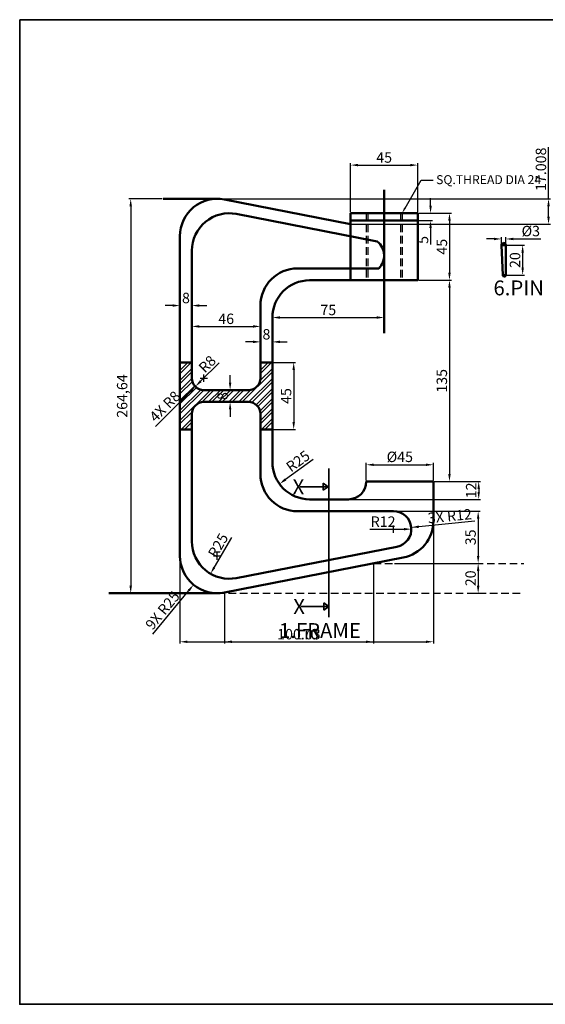
# Model space of a CAD drawing. Units: millimetres. Extents: x 210 to 1120, y -242 to 418.
# Tile 1 of 4: x 210 to 563, y -242 to 418. Entities that reach past the tile are written whole.
import ezdxf
from ezdxf import colors
from ezdxf.entities.mleader import LeaderData, LeaderLine
from ezdxf.math import Vec2, Vec3

# ---------------------------------------------------------------- set-up
doc = ezdxf.new("R2010")
doc.units = ezdxf.units.MM
doc.header["$LTSCALE"] = 0.4
doc.linetypes.add('DASHED', pattern=[19.05, 12.7, -6.35])
for name, color, linetype, lineweight in [('M-DIMS', 2, 'Continuous', 25), ('M-HATC', 8, 'Continuous', 18), ('M-HIDN', 4, 'DASHED', 25), ('M-OUTL', 7, 'Continuous', 50), ('M-SECT', 6, 'Continuous', 35), ('M-TEXT', 3, 'Continuous', 25), ('M-TTLB', 7, 'Continuous', 35)]:
    doc.layers.add(name, color=color, linetype=linetype, lineweight=lineweight)
doc.styles.get("Standard").update_dxf_attribs({"font": 'arial.ttf'})
doc.dimstyles.new('ISO-25', dxfattribs={"dimtxt": 7, "dimasz": 5, "dimexe": 1.25, "dimexo": 0.625, "dimtad": 1, "dimtxsty": 'Standard', "dimcen": 2.5, "dimadec": 0, "dimazin": 0, "dimtfac": 1, "dimtofl": 0, "dimtmove": 0, "dimatfit": 3, "dimfxl": 1, "dimarcsym": 0})

# ---------------------------------------------------------------- blocks, each defined once
blk = doc.blocks.new('*D1')
at = {"layer": 'Defpoints', "color": 0, "transparency": 16777216}
for p in [(350.72, 68.21), (338.22, 46.56)]:
    blk.add_point(p, dxfattribs=at)
at = {"layer": 'M-DIMS', "color": 0, "lineweight": -2, "transparency": 16777216}
blk.add_line((352.23, 70.83), (340.72, 50.89), dxfattribs=at)
at = {"layer": 'M-DIMS', "color": 0, "transparency": 16777216}
blk.add_solid([(340, 51.31), (341.44, 50.47), (338.22, 46.56)], dxfattribs=at)
at = {"layer": 'M-DIMS', "color": 0, "transparency": 16777216, "insert": (344.09, 65.13), "char_height": 7, "attachment_point": 5, "rotation": 60}
blk.add_mtext('R25', dxfattribs=at)
blk = doc.blocks.new('*D2')
at = {"layer": 'Defpoints', "color": 0, "transparency": 16777216}
for p in [(404.72, 121.5), (384.46, 106.85)]:
    blk.add_point(p, dxfattribs=at)
at = {"layer": 'M-DIMS', "color": 0, "lineweight": -2, "transparency": 16777216}
blk.add_line((407.17, 123.27), (388.51, 109.78), dxfattribs=at)
at = {"layer": 'M-DIMS', "color": 0, "transparency": 16777216}
blk.add_solid([(388.02, 110.45), (389, 109.1), (384.46, 106.85)], dxfattribs=at)
at = {"layer": 'M-DIMS', "color": 0, "transparency": 16777216, "insert": (397.41, 121.39), "char_height": 7, "attachment_point": 5, "rotation": 35.87577}
blk.add_mtext('R25', dxfattribs=at)
blk = doc.blocks.new('*D3')
at = {"layer": 'Defpoints', "color": 0, "transparency": 16777216}
for p in [(460.96, 76.5), (472.96, 76.5)]:
    blk.add_point(p, dxfattribs=at)
at = {"layer": 'M-DIMS', "color": 0, "lineweight": -2, "transparency": 16777216}
blk.add_line((445.06, 76.5), (467.96, 76.5), dxfattribs=at)
at = {"layer": 'M-DIMS', "color": 0, "transparency": 16777216}
blk.add_solid([(467.96, 77.33), (467.96, 75.66), (472.96, 76.5)], dxfattribs=at)
at = {"layer": 'M-DIMS', "color": 0, "transparency": 16777216, "insert": (454.01, 80.64), "char_height": 7, "attachment_point": 5}
blk.add_mtext('R12', dxfattribs=at)
blk = doc.blocks.new('*D4')
at = {"layer": 'Defpoints', "color": 0, "transparency": 16777216}
for p in [(328.02, 172.2), (333.72, 177.82)]:
    blk.add_point(p, dxfattribs=at)
at = {"layer": 'M-DIMS', "color": 0, "lineweight": -2, "transparency": 16777216}
blk.add_line((344.08, 188.04), (331.58, 175.71), dxfattribs=at)
at = {"layer": 'M-DIMS', "color": 0, "transparency": 16777216}
blk.add_solid([(331, 176.31), (332.17, 175.12), (328.02, 172.2)], dxfattribs=at)
at = {"layer": 'M-DIMS', "color": 0, "transparency": 16777216, "insert": (336.66, 186.62), "char_height": 7, "attachment_point": 5, "rotation": 44.59101}
blk.add_mtext('R8', dxfattribs=at)
blk = doc.blocks.new('*D5')
at = {"layer": 'Defpoints', "color": 0, "transparency": 16777216}
for p in [(306.33, 298.14), (284.66, 33.5), (306.33, 33.5)]:
    blk.add_point(p, dxfattribs=at)
at = {"layer": 'M-DIMS', "color": 0, "lineweight": -2, "transparency": 16777216}
for p, q in [((305.7, 298.14), (283.41, 298.14)), ((284.66, 293.14), (284.66, 38.5)), ((305.7, 33.5), (283.41, 33.5))]:
    blk.add_line(p, q, dxfattribs=at)
at = {"layer": 'M-DIMS', "color": 0, "transparency": 16777216}
for points in [[(283.82, 293.14), (285.49, 293.14), (284.66, 298.14)], [(283.82, 38.5), (285.49, 38.5), (284.66, 33.5)]]:
    blk.add_solid(points, dxfattribs=at)
at = {"layer": 'M-DIMS', "color": 0, "transparency": 16777216, "insert": (279.82, 165.82), "char_height": 7, "attachment_point": 5, "rotation": 90}
blk.add_mtext('264,64', dxfattribs=at)
blk = doc.blocks.new('*D6')
at = {"layer": 'Defpoints', "color": 0, "transparency": 16777216}
for p in [(317.72, 226.51), (325.72, 226.51), (325.72, 226.51)]:
    blk.add_point(p, dxfattribs=at)
at = {"layer": 'M-DIMS', "color": 0, "lineweight": -2, "transparency": 16777216}
for p, q in [((312.72, 226.51), (307.72, 226.51)), ((317.72, 227.14), (317.72, 227.76)), ((325.72, 227.14), (325.72, 227.76)), ((330.72, 226.51), (335.72, 226.51))]:
    blk.add_line(p, q, dxfattribs=at)
at = {"layer": 'M-DIMS', "color": 0, "transparency": 16777216}
for points in [[(312.72, 227.35), (312.72, 225.68), (317.72, 226.51)], [(330.72, 227.35), (330.72, 225.68), (325.72, 226.51)]]:
    blk.add_solid(points, dxfattribs=at)
at = {"layer": 'M-DIMS', "color": 0, "transparency": 16777216, "insert": (321.72, 230.71), "char_height": 7, "attachment_point": 5}
blk.add_mtext('8', dxfattribs=at)
blk = doc.blocks.new('*D7')
at = {"layer": 'Defpoints', "color": 0, "transparency": 16777216}
for p in [(371.72, 212.54), (325.72, 209.96), (371.72, 209.96)]:
    blk.add_point(p, dxfattribs=at)
at = {"layer": 'M-DIMS', "color": 0, "lineweight": -2, "transparency": 16777216}
for p, q in [((325.72, 210.58), (325.72, 213.79)), ((330.72, 212.54), (366.72, 212.54)), ((371.72, 210.58), (371.72, 213.79))]:
    blk.add_line(p, q, dxfattribs=at)
at = {"layer": 'M-DIMS', "color": 0, "transparency": 16777216}
for points in [[(330.72, 213.37), (330.72, 211.7), (325.72, 212.54)], [(366.72, 213.37), (366.72, 211.7), (371.72, 212.54)]]:
    blk.add_solid(points, dxfattribs=at)
at = {"layer": 'M-DIMS', "color": 0, "transparency": 16777216, "insert": (348.72, 216.74), "char_height": 7, "attachment_point": 5}
blk.add_mtext('46', dxfattribs=at)
blk = doc.blocks.new('*D8')
at = {"layer": 'Defpoints', "color": 0, "transparency": 16777216}
for p in [(371.72, 202.16), (379.72, 202.16), (379.72, 202.16)]:
    blk.add_point(p, dxfattribs=at)
at = {"layer": 'M-DIMS', "color": 0, "lineweight": -2, "transparency": 16777216}
for p, q in [((366.72, 202.16), (361.72, 202.16)), ((371.72, 202.78), (371.72, 203.41)), ((379.72, 202.78), (379.72, 203.41)), ((384.72, 202.16), (389.72, 202.16))]:
    blk.add_line(p, q, dxfattribs=at)
at = {"layer": 'M-DIMS', "color": 0, "transparency": 16777216}
for points in [[(366.72, 202.99), (366.72, 201.33), (371.72, 202.16)], [(384.72, 202.99), (384.72, 201.33), (379.72, 202.16)]]:
    blk.add_solid(points, dxfattribs=at)
at = {"layer": 'M-DIMS', "color": 0, "transparency": 16777216, "insert": (375.72, 206.36), "char_height": 7, "attachment_point": 5}
blk.add_mtext('8', dxfattribs=at)
blk = doc.blocks.new('*D9')
at = {"layer": 'Defpoints', "color": 0, "transparency": 16777216}
for p in [(379.72, 188.32), (379.72, 143.32), (394.01, 143.32)]:
    blk.add_point(p, dxfattribs=at)
at = {"layer": 'M-DIMS', "color": 0, "lineweight": -2, "transparency": 16777216}
for p, q in [((380.34, 188.32), (395.26, 188.32)), ((394.01, 183.32), (394.01, 148.32)), ((380.34, 143.32), (395.26, 143.32))]:
    blk.add_line(p, q, dxfattribs=at)
at = {"layer": 'M-DIMS', "color": 0, "transparency": 16777216}
for points in [[(393.18, 183.32), (394.85, 183.32), (394.01, 188.32)], [(393.18, 148.32), (394.85, 148.32), (394.01, 143.32)]]:
    blk.add_solid(points, dxfattribs=at)
at = {"layer": 'M-DIMS', "color": 0, "transparency": 16777216, "insert": (389.83, 165.82), "char_height": 7, "attachment_point": 5, "rotation": 90}
blk.add_mtext('45', dxfattribs=at)
blk = doc.blocks.new('*D10')
at = {"layer": 'Defpoints', "color": 0, "transparency": 16777216}
for p in [(348.72, 169.82), (348.72, 161.82), (351.36, 161.82)]:
    blk.add_point(p, dxfattribs=at)
at = {"layer": 'M-DIMS', "color": 0, "lineweight": -2, "transparency": 16777216}
for p, q in [((351.36, 174.82), (351.36, 179.82)), ((349.34, 169.82), (352.61, 169.82)), ((349.34, 161.82), (352.61, 161.82)), ((351.36, 156.82), (351.36, 151.82))]:
    blk.add_line(p, q, dxfattribs=at)
at = {"layer": 'M-DIMS', "color": 0, "transparency": 16777216}
for points in [[(350.52, 174.82), (352.19, 174.82), (351.36, 169.82)], [(350.52, 156.82), (352.19, 156.82), (351.36, 161.82)]]:
    blk.add_solid(points, dxfattribs=at)
at = {"layer": 'M-DIMS', "color": 0, "transparency": 16777216, "insert": (347.16, 165.82), "char_height": 7, "attachment_point": 5, "rotation": 90}
blk.add_mtext('8', dxfattribs=at)
blk = doc.blocks.new('*D11')
at = {"layer": 'Defpoints', "color": 0, "transparency": 16777216}
for p in [(379.72, 218.5), (454.72, 218.5), (454.72, 218.5)]:
    blk.add_point(p, dxfattribs=at)
at = {"layer": 'M-DIMS', "color": 0, "lineweight": -2, "transparency": 16777216}
for p, q in [((379.72, 219.12), (379.72, 219.75)), ((384.72, 218.5), (449.72, 218.5)), ((454.72, 219.12), (454.72, 219.75))]:
    blk.add_line(p, q, dxfattribs=at)
at = {"layer": 'M-DIMS', "color": 0, "transparency": 16777216}
for points in [[(384.72, 219.33), (384.72, 217.66), (379.72, 218.5)], [(449.72, 219.33), (449.72, 217.66), (454.72, 218.5)]]:
    blk.add_solid(points, dxfattribs=at)
at = {"layer": 'M-DIMS', "color": 0, "transparency": 16777216, "insert": (417.22, 222.68), "char_height": 7, "attachment_point": 5}
blk.add_mtext('75', dxfattribs=at)
blk = doc.blocks.new('*D12')
at = {"layer": 'Defpoints', "color": 0, "transparency": 16777216}
for p in [(477.22, 288.5), (477.22, 243.5), (498.54, 243.5)]:
    blk.add_point(p, dxfattribs=at)
at = {"layer": 'M-DIMS', "color": 0, "lineweight": -2, "transparency": 16777216}
for p, q in [((477.84, 288.5), (499.79, 288.5)), ((498.54, 283.5), (498.54, 248.5)), ((477.84, 243.5), (499.79, 243.5))]:
    blk.add_line(p, q, dxfattribs=at)
at = {"layer": 'M-DIMS', "color": 0, "transparency": 16777216}
for points in [[(497.7, 283.5), (499.37, 283.5), (498.54, 288.5)], [(497.7, 248.5), (499.37, 248.5), (498.54, 243.5)]]:
    blk.add_solid(points, dxfattribs=at)
at = {"layer": 'M-DIMS', "color": 0, "transparency": 16777216, "insert": (494.35, 266), "char_height": 7, "attachment_point": 5, "rotation": 90}
blk.add_mtext('45', dxfattribs=at)
blk = doc.blocks.new('*D13')
at = {"layer": 'Defpoints', "color": 0, "transparency": 16777216}
for p in [(487.72, 119.69), (442.72, 108.5), (487.72, 108.5)]:
    blk.add_point(p, dxfattribs=at)
at = {"layer": 'M-DIMS', "color": 0, "lineweight": -2, "transparency": 16777216}
for p, q in [((442.72, 109.12), (442.72, 120.94)), ((447.72, 119.69), (482.72, 119.69)), ((487.72, 109.12), (487.72, 120.94))]:
    blk.add_line(p, q, dxfattribs=at)
at = {"layer": 'M-DIMS', "color": 0, "transparency": 16777216}
for points in [[(447.72, 120.52), (447.72, 118.86), (442.72, 119.69)], [(482.72, 120.52), (482.72, 118.86), (487.72, 119.69)]]:
    blk.add_solid(points, dxfattribs=at)
at = {"layer": 'M-DIMS', "color": 0, "transparency": 16777216, "insert": (465.22, 124.09), "char_height": 7, "attachment_point": 5}
blk.add_mtext('%%C45', dxfattribs=at)
blk = doc.blocks.new('*D14')
at = {"layer": 'Defpoints', "color": 0, "transparency": 16777216}
for p in [(487.72, 108.5), (417.72, 96.5), (518.15, 96.5)]:
    blk.add_point(p, dxfattribs=at)
at = {"layer": 'M-DIMS', "color": 0, "lineweight": -2, "transparency": 16777216}
for p, q in [((488.34, 108.5), (519.4, 108.5)), ((518.15, 103.5), (518.15, 101.5)), ((418.34, 96.5), (519.4, 96.5))]:
    blk.add_line(p, q, dxfattribs=at)
at = {"layer": 'M-DIMS', "color": 0, "transparency": 16777216}
for points in [[(517.32, 103.5), (518.98, 103.5), (518.15, 108.5)], [(517.32, 101.5), (518.98, 101.5), (518.15, 96.5)]]:
    blk.add_solid(points, dxfattribs=at)
at = {"layer": 'M-DIMS', "color": 0, "transparency": 16777216, "insert": (514.01, 102.5), "char_height": 7, "attachment_point": 5, "rotation": 90}
blk.add_mtext('12', dxfattribs=at)
blk = doc.blocks.new('*D15')
at = {"layer": 'Defpoints', "color": 0, "transparency": 16777216}
for p in [(511.06, 53.5), (511.06, 33.5), (517.8, 33.5)]:
    blk.add_point(p, dxfattribs=at)
at = {"layer": 'M-DIMS', "color": 0, "lineweight": -2, "transparency": 16777216}
for p, q in [((511.68, 53.5), (519.05, 53.5)), ((517.8, 48.5), (517.8, 38.5)), ((511.68, 33.5), (519.05, 33.5))]:
    blk.add_line(p, q, dxfattribs=at)
at = {"layer": 'M-DIMS', "color": 0, "transparency": 16777216}
for points in [[(516.96, 48.5), (518.63, 48.5), (517.8, 53.5)], [(516.96, 38.5), (518.63, 38.5), (517.8, 33.5)]]:
    blk.add_solid(points, dxfattribs=at)
at = {"layer": 'M-DIMS', "color": 0, "transparency": 16777216, "insert": (513.6, 43.5), "char_height": 7, "attachment_point": 5, "rotation": 90}
blk.add_mtext('20', dxfattribs=at)
blk = doc.blocks.new('*D16')
at = {"layer": 'Defpoints', "color": 0, "transparency": 16777216}
for p in [(460.96, 88.5), (460.96, 53.5), (517.8, 53.5)]:
    blk.add_point(p, dxfattribs=at)
at = {"layer": 'M-DIMS', "color": 0, "lineweight": -2, "transparency": 16777216}
for p, q in [((461.59, 88.5), (519.05, 88.5)), ((517.8, 83.5), (517.8, 58.5)), ((461.59, 53.5), (519.05, 53.5))]:
    blk.add_line(p, q, dxfattribs=at)
at = {"layer": 'M-DIMS', "color": 0, "transparency": 16777216}
for points in [[(516.96, 83.5), (518.63, 83.5), (517.8, 88.5)], [(516.96, 58.5), (518.63, 58.5), (517.8, 53.5)]]:
    blk.add_solid(points, dxfattribs=at)
at = {"layer": 'M-DIMS', "color": 0, "transparency": 16777216, "insert": (513.6, 71), "char_height": 7, "attachment_point": 5, "rotation": 90}
blk.add_mtext('35', dxfattribs=at)
blk = doc.blocks.new('*D17')
at = {"layer": 'Defpoints', "color": 0, "transparency": 16777216}
for p in [(488.81, 243.5), (488.81, 108.5), (498.54, 108.5)]:
    blk.add_point(p, dxfattribs=at)
at = {"layer": 'M-DIMS', "color": 0, "lineweight": -2, "transparency": 16777216}
for p, q in [((489.44, 243.5), (499.79, 243.5)), ((498.54, 238.5), (498.54, 113.5)), ((489.44, 108.5), (499.79, 108.5))]:
    blk.add_line(p, q, dxfattribs=at)
at = {"layer": 'M-DIMS', "color": 0, "transparency": 16777216}
for points in [[(497.7, 238.5), (499.37, 238.5), (498.54, 243.5)], [(497.7, 113.5), (499.37, 113.5), (498.54, 108.5)]]:
    blk.add_solid(points, dxfattribs=at)
at = {"layer": 'M-DIMS', "color": 0, "transparency": 16777216, "insert": (494.33, 176), "char_height": 7, "attachment_point": 5, "rotation": 90}
blk.add_mtext('135', dxfattribs=at)
blk = doc.blocks.new('*D20')
at = {"layer": 'Defpoints', "color": 0, "transparency": 16777216}
for p in [(477.22, 288.5), (477.22, 283.5), (485.85, 283.5)]:
    blk.add_point(p, dxfattribs=at)
at = {"layer": 'M-DIMS', "color": 0, "lineweight": -2, "transparency": 16777216}
for p, q in [((485.85, 293.5), (485.85, 298.5)), ((477.84, 288.5), (487.1, 288.5)), ((477.84, 283.5), (487.1, 283.5)), ((485.85, 278.5), (485.85, 267.61))]:
    blk.add_line(p, q, dxfattribs=at)
at = {"layer": 'M-DIMS', "color": 0, "transparency": 16777216}
for points in [[(485.02, 293.5), (486.68, 293.5), (485.85, 288.5)], [(485.02, 278.5), (486.68, 278.5), (485.85, 283.5)]]:
    blk.add_solid(points, dxfattribs=at)
at = {"layer": 'M-DIMS', "color": 0, "transparency": 16777216, "insert": (481.67, 270.55), "char_height": 7, "attachment_point": 5, "rotation": 90}
blk.add_mtext('5', dxfattribs=at)
blk = doc.blocks.new('*D43')
at = {"layer": 'Defpoints', "color": 0, "ltscale": 0.4, "transparency": 16777216}
for p in [(534.88, 267.02), (535.38, 247.02), (547.64, 247.02)]:
    blk.add_point(p, dxfattribs=at)
at = {"layer": 'M-DIMS', "color": 0, "lineweight": -2, "ltscale": 0.4, "transparency": 16777216}
for p, q in [((535.51, 267.02), (548.89, 267.02)), ((547.64, 262.02), (547.64, 252.02)), ((536.01, 247.02), (548.89, 247.02))]:
    blk.add_line(p, q, dxfattribs=at)
at = {"layer": 'M-DIMS', "color": 0, "ltscale": 0.4, "transparency": 16777216}
for points in [[(546.81, 262.02), (548.48, 262.02), (547.64, 267.02)], [(546.81, 252.02), (548.48, 252.02), (547.64, 247.02)]]:
    blk.add_solid(points, dxfattribs=at)
at = {"layer": 'M-DIMS', "color": 0, "ltscale": 0.4, "transparency": 16777216, "insert": (543.44, 257.02), "char_height": 7, "attachment_point": 5, "rotation": 90}
blk.add_mtext('20', dxfattribs=at)
blk = doc.blocks.new('*D44')
at = {"layer": 'Defpoints', "color": 0, "ltscale": 0.4, "transparency": 16777216}
for p in [(536.38, 271.22), (533.38, 267.02), (536.38, 267.02)]:
    blk.add_point(p, dxfattribs=at)
at = {"layer": 'M-DIMS', "color": 0, "lineweight": -2, "ltscale": 0.4, "transparency": 16777216}
for p, q in [((528.38, 271.22), (523.38, 271.22)), ((533.38, 267.65), (533.38, 272.47)), ((536.38, 267.65), (536.38, 272.47)), ((541.38, 271.22), (559.84, 271.22))]:
    blk.add_line(p, q, dxfattribs=at)
at = {"layer": 'M-DIMS', "color": 0, "ltscale": 0.4, "transparency": 16777216}
for points in [[(528.38, 272.05), (528.38, 270.38), (533.38, 271.22)], [(541.38, 272.05), (541.38, 270.38), (536.38, 271.22)]]:
    blk.add_solid(points, dxfattribs=at)
at = {"layer": 'M-DIMS', "color": 0, "ltscale": 0.4, "transparency": 16777216, "insert": (553.11, 275.61), "char_height": 7, "attachment_point": 5}
blk.add_mtext('%%C3', dxfattribs=at)
blk = doc.blocks.new('SECTION-ARROW')
for p, q in [((0, 2.43), (18.69, 2.43)), ((15.48, 2.43), (15.48, 4.85)), ((15.48, 4.85), (18.69, 2.43)), ((15.48, 2.43), (15.48, 0)), ((15.48, 0), (18.69, 2.43))]:
    blk.add_line(p, q)
blk = doc.blocks.new('*D46')
at = {"layer": 'Defpoints', "color": 0, "ltscale": 0.4, "transparency": 16777216}
for p in [(487.72, 108.5), (317.72, 58.5), (487.72, 0.92)]:
    blk.add_point(p, dxfattribs=at)
at = {"layer": 'M-DIMS', "color": 0, "lineweight": -2, "ltscale": 0.4, "transparency": 16777216}
for p, q in [((487.72, 107.87), (487.72, -0.33)), ((317.72, 57.87), (317.72, -0.33)), ((322.72, 0.92), (482.72, 0.92))]:
    blk.add_line(p, q, dxfattribs=at)
at = {"layer": 'M-DIMS', "color": 0, "ltscale": 0.4, "transparency": 16777216}
for points in [[(322.72, 1.75), (322.72, 0.08), (317.72, 0.92)], [(482.72, 1.75), (482.72, 0.08), (487.72, 0.92)]]:
    blk.add_solid(points, dxfattribs=at)
at = {"layer": 'M-DIMS', "color": 0, "ltscale": 0.4, "transparency": 16777216, "insert": (402.72, 5.12), "char_height": 7, "attachment_point": 5}
blk.add_mtext('170', dxfattribs=at)
blk = doc.blocks.new('*D47')
at = {"layer": 'Defpoints', "color": 0, "ltscale": 0.4, "transparency": 16777216}
for p in [(477.22, 320.78), (432.22, 288.5), (477.22, 288.5)]:
    blk.add_point(p, dxfattribs=at)
at = {"layer": 'M-DIMS', "color": 0, "lineweight": -2, "ltscale": 0.4, "transparency": 16777216}
for p, q in [((432.22, 289.12), (432.22, 322.03)), ((437.22, 320.78), (472.22, 320.78)), ((477.22, 289.12), (477.22, 322.03))]:
    blk.add_line(p, q, dxfattribs=at)
at = {"layer": 'M-DIMS', "color": 0, "ltscale": 0.4, "transparency": 16777216}
for points in [[(437.22, 321.62), (437.22, 319.95), (432.22, 320.78)], [(472.22, 321.62), (472.22, 319.95), (477.22, 320.78)]]:
    blk.add_solid(points, dxfattribs=at)
at = {"layer": 'M-DIMS', "color": 0, "ltscale": 0.4, "transparency": 16777216, "insert": (454.72, 324.97), "char_height": 7, "attachment_point": 5}
blk.add_mtext('45', dxfattribs=at)
blk = doc.blocks.new('*D48')
at = {"layer": 'Defpoints', "color": 0, "ltscale": 0.4, "transparency": 16777216}
for p in [(342.72, 298.14), (565, 298.14), (432.22, 281.13)]:
    blk.add_point(p, dxfattribs=at)
at = {"layer": 'M-DIMS', "color": 0, "lineweight": -2, "ltscale": 0.4, "transparency": 16777216}
for p, q in [((565, 298.14), (565, 332.81)), ((343.34, 298.14), (566.25, 298.14)), ((565, 286.13), (565, 293.14)), ((432.84, 281.13), (566.25, 281.13))]:
    blk.add_line(p, q, dxfattribs=at)
at = {"layer": 'M-DIMS', "color": 0, "ltscale": 0.4, "transparency": 16777216}
for points in [[(564.16, 293.14), (565.83, 293.14), (565, 298.14)], [(564.16, 286.13), (565.83, 286.13), (565, 281.13)]]:
    blk.add_solid(points, dxfattribs=at)
at = {"layer": 'M-DIMS', "color": 0, "ltscale": 0.4, "transparency": 16777216, "insert": (560.8, 317.98), "char_height": 7, "attachment_point": 5, "rotation": 90}
blk.add_mtext('17.008', dxfattribs=at)
blk = doc.blocks.new('*D49')
at = {"layer": 'Defpoints', "color": 0, "ltscale": 0.4, "transparency": 16777216}
for p in [(447.54, 53.5), (347.51, 33.96), (447.54, 0.92)]:
    blk.add_point(p, dxfattribs=at)
at = {"layer": 'M-DIMS', "color": 0, "lineweight": -2, "ltscale": 0.4, "transparency": 16777216}
for p, q in [((447.54, 52.87), (447.54, -0.33)), ((347.51, 33.34), (347.51, -0.33)), ((352.51, 0.92), (442.54, 0.92))]:
    blk.add_line(p, q, dxfattribs=at)
at = {"layer": 'M-DIMS', "color": 0, "ltscale": 0.4, "transparency": 16777216}
for points in [[(352.51, 1.75), (352.51, 0.08), (347.51, 0.92)], [(442.54, 1.75), (442.54, 0.08), (447.54, 0.92)]]:
    blk.add_solid(points, dxfattribs=at)
at = {"layer": 'M-DIMS', "color": 0, "ltscale": 0.4, "transparency": 16777216, "insert": (397.52, 5.12), "char_height": 7, "attachment_point": 5}
blk.add_mtext('100.03', dxfattribs=at)
blk = doc.blocks.new('*D54')
at = {"layer": 'Defpoints', "color": 0, "ltscale": 0.4, "transparency": 16777216}
for p in [(342.72, 58.5), (326.83, 39.2)]:
    blk.add_point(p, dxfattribs=at)
at = {"layer": 'M-DIMS', "color": 0, "lineweight": -2, "ltscale": 0.4, "transparency": 16777216}
for p, q in [((342.72, 56), (342.72, 61)), ((340.22, 58.5), (345.22, 58.5)), ((299.45, 5.95), (323.65, 35.34))]:
    blk.add_line(p, q, dxfattribs=at)
at = {"layer": 'M-DIMS', "color": 0, "ltscale": 0.4, "transparency": 16777216}
blk.add_solid([(323, 35.87), (324.29, 34.81), (326.83, 39.2)], dxfattribs=at)
at = {"layer": 'M-DIMS', "color": 0, "ltscale": 0.4, "transparency": 16777216, "insert": (306.72, 21.39), "char_height": 7, "attachment_point": 5, "rotation": 50.52629}
blk.add_mtext('9X R25', dxfattribs=at)
blk = doc.blocks.new('*D55')
at = {"layer": 'Defpoints', "color": 0, "ltscale": 0.4, "transparency": 16777216}
for p in [(460.96, 76.5), (472.91, 77.65)]:
    blk.add_point(p, dxfattribs=at)
at = {"layer": 'M-DIMS', "color": 0, "lineweight": -2, "ltscale": 0.4, "transparency": 16777216}
for p, q in [((515.65, 81.79), (477.88, 78.13)), ((458.46, 76.5), (463.46, 76.5)), ((460.96, 74), (460.96, 79))]:
    blk.add_line(p, q, dxfattribs=at)
at = {"layer": 'M-DIMS', "color": 0, "ltscale": 0.4, "transparency": 16777216}
blk.add_solid([(477.8, 78.96), (477.96, 77.3), (472.91, 77.65)], dxfattribs=at)
at = {"layer": 'M-DIMS', "color": 0, "ltscale": 0.4, "transparency": 16777216, "insert": (498.85, 84.38), "char_height": 7, "attachment_point": 5, "rotation": 5.52485}
blk.add_mtext('3X R12', dxfattribs=at)
blk = doc.blocks.new('*D56')
at = {"layer": 'Defpoints', "color": 0, "ltscale": 0.4, "transparency": 16777216}
for p in [(328.06, 172.16), (333.72, 177.82)]:
    blk.add_point(p, dxfattribs=at)
at = {"layer": 'M-DIMS', "color": 0, "lineweight": -2, "ltscale": 0.4, "transparency": 16777216}
for p, q in [((333.72, 175.32), (333.72, 180.32)), ((331.22, 177.82), (336.22, 177.82)), ((301.28, 145.38), (324.53, 168.63))]:
    blk.add_line(p, q, dxfattribs=at)
at = {"layer": 'M-DIMS', "color": 0, "ltscale": 0.4, "transparency": 16777216}
blk.add_solid([(323.94, 169.22), (325.12, 168.04), (328.06, 172.16)], dxfattribs=at)
at = {"layer": 'M-DIMS', "color": 0, "ltscale": 0.4, "transparency": 16777216, "insert": (308.17, 158.21), "char_height": 7, "attachment_point": 5, "rotation": 45.00087}
blk.add_mtext('4X R8', dxfattribs=at)

msp = doc.modelspace()

# ---------------------------------------------------------------- hatches: boundary and pattern name
at = {"layer": 'M-HATC'}
h = msp.add_hatch(dxfattribs=at)
h.set_pattern_fill('ANSI32', color=256, scale=0.5)
h.paths.add_polyline_path([(379.7189, 188.3201), (371.7189, 188.3201), (371.7189, 177.8201, -0.41421356), (363.7189, 169.8201), (333.7189, 169.8201, -0.41421356), (325.7189, 177.8201), (325.7189, 188.3201), (317.7189, 188.3201), (317.7189, 165.8201), (317.7189, 143.3201), (325.7189, 143.3201), (325.7189, 153.8201, -0.41421356), (333.7189, 161.8201), (363.7189, 161.8201, -0.41421356), (371.7189, 153.8201), (371.7189, 143.3201), (379.7189, 143.3201), (379.7189, 165.8201)])

# ---------------------------------------------------------------- linework, layer by layer
at = {"layer": 'M-HIDN'}
for p, q in [((442.7189, 288.4977), (442.7189, 243.4977)), ((443.7189, 288.4977), (443.7189, 243.4977)), ((465.7189, 288.4977), (465.7189, 243.4977)), ((466.7189, 288.4977), (466.7189, 243.4977)), ((447.5374, 53.4977), (548.4982, 53.4977)), ((342.7189, 33.4977), (548.3926, 33.4977))]:
    msp.add_line(p, q, dxfattribs=at)
at = {"layer": 'M-OUTL'}
for p, q in [((454.7189, 208.0107), (454.7189, 304.2823)), ((342.7189, 298.1425), (306.3276, 298.1425)), ((432.2189, 281.1344), (347.5112, 297.6789)), ((450.1236, 269.4862), (355.5112, 287.9652)), ((477.2189, 288.4977), (432.2189, 288.4977)), ((432.2189, 288.4977), (432.2189, 243.4977)), ((454.7189, 288.4977), (454.7189, 243.4977)), ((477.2189, 243.4977), (477.2189, 288.4977)), ((477.2189, 283.4977), (432.2189, 283.4977)), ((454.7189, 278.4977), (454.7189, 283.4977)), ((317.7189, 165.8201), (317.7189, 273.1425)), ((325.7189, 177.8201), (325.7189, 263.4288)), ((396.7189, 251.4977), (451.1435, 251.4977)), ((404.7189, 243.4977), (477.2189, 243.4977)), ((432.2189, 243.4977), (477.2189, 243.4977)), ((371.7189, 177.8201), (371.7189, 226.4977)), ((379.7189, 165.8201), (379.7189, 218.4977)), ((317.7189, 188.3201), (325.7189, 188.3201)), ((371.7189, 188.3201), (379.7189, 188.3201)), ((317.7189, 165.8201), (317.7189, 58.4977)), ((333.7189, 169.8201), (363.7189, 169.8201)), ((379.7189, 165.8201), (379.7189, 121.4977)), ((333.7189, 161.8201), (363.7189, 161.8201)), ((325.7189, 153.8201), (325.7189, 68.2113)), ((371.7189, 153.8201), (371.7189, 113.4977)), ((317.7189, 143.3201), (325.7189, 143.3201)), ((371.7189, 143.3201), (379.7189, 143.3201)), ((442.7189, 108.4977), (487.7189, 108.4977)), ((487.7189, 81.9352), (487.7189, 108.4977)), ((404.7189, 96.4977), (430.7189, 96.4977)), ((396.7189, 88.4977), (460.9626, 88.4977)), ((463.2629, 64.7202), (355.5112, 43.6749)), ((467.5112, 57.3988), (347.5112, 33.9613)), ((342.7189, 33.4977), (270.0229, 33.4977))]:
    msp.add_line(p, q, dxfattribs=at)
at = {"layer": 'M-OUTL', "ltscale": 0.4}
for p, q in [((536.3815, 267.0225), (533.3815, 267.0225)), ((534.3815, 247.0225), (533.3815, 267.0225)), ((536.3815, 267.0225), (536.3815, 247.0225)), ((536.3815, 247.0225), (534.3815, 247.0225))]:
    msp.add_line(p, q, dxfattribs=at)
at = {"layer": 'M-OUTL'}
for centre, radius, start, end in [((342.7189, 273.1425), 25, 78.948543, 180), ((350.7189, 263.4288), 25, 78.948543, 180), ((442.7189, 260.0432), 12, 314.5918306, 51.8986166), ((396.7189, 226.4977), 25, 90, 180), ((404.7189, 218.4977), 25, 90, 180), ((333.7189, 177.8201), 8, 180, 270), ((363.7189, 177.8201), 8, 270, 0), ((333.7189, 153.8201), 8, 90, 180), ((363.7189, 153.8201), 8, 0, 90), ((404.7189, 121.4977), 25, 180, 270), ((396.7189, 113.4977), 25, 180, 270), ((430.7189, 108.4977), 12, 270, 360), ((460.9626, 76.4977), 12, 281.051457, 90), ((462.7189, 81.9352), 25, 281.051457, 0), ((350.7189, 68.2113), 25, 180, 281.051457), ((342.7189, 58.4977), 25, 180, 281.051457)]:
    msp.add_arc(centre, radius, start, end, dxfattribs=at)
at = {"layer": 'M-OUTL', "ltscale": 0.4}
for centre, radius, start, end in [((534.8815, 267.0225), 1.5, 0, 185.7248105), ((535.3815, 247.0225), 1, 180, 0)]:
    msp.add_arc(centre, radius, start, end, dxfattribs=at)
at = {"layer": 'M-SECT'}
msp.add_line((417.5578, 117.2772), (417.5578, 17.4177), dxfattribs=at)
at = {"layer": 'M-TTLB', "ltscale": 0.4}
msp.add_lwpolyline([(210.1659, 418.3486), (1119.5264, 418.3486), (1119.5264, -242.3444), (210.1659, -242.3444)], close=True, dxfattribs=at)

# ---------------------------------------------------------------- block references
at = {"layer": 'M-SECT'}
for p in [(398.3688, 102.5602), (398.863, 22.225)]:
    msp.add_blockref('SECTION-ARROW', p, dxfattribs=at)

# ---------------------------------------------------------------- texts
at = {"layer": 'M-TEXT', "attachment_point": 1}
for s, width, insert, char_height in [('\\pxqc;{\\H0.66667x;6.PIN} ', 102.502816, (493.7359, 243.3752), 15), ('X', 4.451993, (393.2632, 109.8473), 10), ('X', 4.451993, (393.7574, 29.5121), 10), ('\\pxqc;{\\H0.66667x;1.FRAME} ', 159.738723, (331.7515, 13.4299), 15)]:
    msp.add_mtext_dynamic_manual_height_columns(s, width=width, gutter_width=12.5, heights=[0], dxfattribs=dict(at, insert=insert, char_height=char_height))

# ---------------------------------------------------------------- dimensions: what is measured, and where the dimension line sits
at = {"layer": 'M-DIMS', "ltscale": 0.4}
for base, p1, p2, override, picture, middle in [((564.9982, 298.1425), (432.2189, 281.1344), (342.7189, 298.1425), {"dimdec": 3, "dimlfac": 1, "dimrnd": 0, "dimzin": 0, "dimdsep": 46, "dimlunit": 2}, '*D48', (560.7991, 317.9752)), ((547.642, 247.0225), (534.8815, 267.0225), (535.3815, 247.0225), {"dimclrd": 0, "dimclre": 0, "dimclrt": 0}, '*D43', (543.443, 257.0225))]:
    dim = msp.add_linear_dim(base=base, p1=p1, p2=p2, angle=90, dimstyle='ISO-25', override=override, dxfattribs=at)
    dim.commit()
    dim.dimension.update_dxf_attribs({"geometry": picture, "text_midpoint": middle})
for base, p1, p2, override, picture, middle in [((477.2189, 320.7823), (432.2189, 288.4977), (477.2189, 288.4977), {"dimdec": 0, "dimlfac": 1, "dimrnd": 0, "dimzin": 0, "dimdsep": 46, "dimlunit": 2}, '*D47', (454.7189, 324.967)), ((487.7189, 0.9177), (317.7189, 58.4977), (487.7189, 108.4977), {"dimdec": 0, "dimlfac": 1, "dimrnd": 0, "dimzin": 0, "dimdsep": 46, "dimlunit": 2}, '*D46', (402.7189, 5.1167)), ((447.5374, 0.9177), (347.5112, 33.9613), (447.5374, 53.4977), {"dimdec": 2, "dimlfac": 1, "dimrnd": 0, "dimzin": 0, "dimdsep": 46, "dimlunit": 2}, '*D49', (397.5243, 5.1191))]:
    dim = msp.add_linear_dim(base=base, p1=p1, p2=p2, dimstyle='ISO-25', override=override, dxfattribs=at)
    dim.commit()
    dim.dimension.update_dxf_attribs({"geometry": picture, "text_midpoint": middle})
at = {"layer": 'M-DIMS'}
for base, p1, p2, picture, middle in [((284.6552, 33.4977), (306.3276, 298.1425), (306.3276, 33.4977), '*D5', (279.8236, 165.8201)), ((485.8513, 283.4977), (477.2189, 288.4977), (477.2189, 283.4977), '*D20', (481.6666, 270.5521)), ((498.5354, 243.4977), (477.2189, 288.4977), (477.2189, 243.4977), '*D12', (494.3507, 265.9977)), ((498.5354, 108.4977), (488.8146, 243.4977), (488.8146, 108.4977), '*D17', (494.334, 175.9977)), ((394.0146, 143.3201), (379.7189, 188.3201), (379.7189, 143.3201), '*D9', (389.8299, 165.8201)), ((351.3552, 161.8201), (348.7189, 169.8201), (348.7189, 161.8201), '*D10', (347.1562, 165.8201)), ((518.1515, 96.4977), (487.7189, 108.4977), (417.7189, 96.4977), '*D14', (514.0122, 102.4977)), ((517.7965, 53.4977), (460.9626, 88.4977), (460.9626, 53.4977), '*D16', (513.5951, 70.9977)), ((517.7965, 33.4977), (511.0593, 53.4977), (511.0593, 33.4977), '*D15', (513.5975, 43.4977))]:
    dim = msp.add_linear_dim(base=base, p1=p1, p2=p2, angle=90, dimstyle='ISO-25', override={"dimclrd": 0, "dimclre": 0, "dimclrt": 0}, dxfattribs=at)
    dim.commit()
    dim.dimension.update_dxf_attribs({"geometry": picture, "text_midpoint": middle})
at = {"layer": 'M-DIMS', "ltscale": 0.4}
dim = msp.add_linear_dim(base=(536.3815, 271.2179), p1=(533.3815, 267.0225), p2=(536.3815, 267.0225), text='%%C<>', dimstyle='ISO-25', override={"dimclrd": 0, "dimclre": 0, "dimclrt": 0}, dxfattribs=at)
dim.commit()
dim.dimension.update_dxf_attribs({"geometry": '*D44', "text_midpoint": (553.1088, 275.6127)})
at = {"layer": 'M-DIMS'}
for base, p1, p2, picture, middle in [((325.7189, 226.5129), (317.7189, 226.5129), (325.7189, 226.5129), '*D6', (321.7189, 230.712)), ((454.7189, 218.4977), (379.7189, 218.4977), (454.7189, 218.4977), '*D11', (417.2189, 222.6823)), ((371.7189, 212.5368), (325.7189, 209.9566), (371.7189, 209.9566), '*D7', (348.7189, 216.7359)), ((379.7189, 202.1589), (371.7189, 202.1589), (379.7189, 202.1589), '*D8', (375.7189, 206.3579))]:
    dim = msp.add_linear_dim(base=base, p1=p1, p2=p2, dimstyle='ISO-25', override={"dimclrd": 0, "dimclre": 0, "dimclrt": 0}, dxfattribs=at)
    dim.commit()
    dim.dimension.update_dxf_attribs({"geometry": picture, "text_midpoint": middle})
for center, mpoint, picture, middle in [((333.7189, 177.8201), (328.0218, 172.2037), '*D4', (339.6126, 183.6302)), ((404.7189, 121.4977), (384.4617, 106.8469), '*D2', (399.8689, 117.99)), ((460.9626, 76.4977), (472.9626, 76.4977), '*D3', (454.0102, 76.4977)), ((350.7189, 68.2113), (338.2189, 46.5607), '*D1', (347.7261, 63.0277))]:
    dim = msp.add_radius_dim(center=center, mpoint=mpoint, dimstyle='ISO-25', override={"dimclrd": 0, "dimclre": 0, "dimclrt": 0}, dxfattribs=at)
    dim.commit()
    dim.dimension.update_dxf_attribs({"geometry": picture, "text_midpoint": middle, "dimtype": 164})
at = {"layer": 'M-DIMS', "ltscale": 0.4}
for center, mpoint, text, picture, middle in [((333.7189, 177.8201), (328.0621, 172.1631), '4X <>', '*D56', (308.1669, 158.2057)), ((460.9626, 76.4977), (472.9069, 77.653), '3X <>', '*D55', (498.8499, 84.3834)), ((342.7189, 58.4977), (326.8258, 39.1997), '9X <>', '*D54', (306.7156, 21.3864))]:
    dim = msp.add_radius_dim(center=center, mpoint=mpoint, text=text, dimstyle='ISO-25', override={"dimdec": 0, "dimlfac": 1, "dimrnd": 0, "dimzin": 0, "dimdsep": 46, "dimlunit": 2}, dxfattribs=at)
    dim.commit()
    dim.dimension.update_dxf_attribs({"geometry": picture, "text_midpoint": middle})
at = {"layer": 'M-DIMS'}
dim = msp.add_linear_dim(base=(487.7189, 119.6906), p1=(442.7189, 108.4977), p2=(487.7189, 108.4977), text='%%C<>', dimstyle='ISO-25', override={"dimclrd": 0, "dimclre": 0, "dimclrt": 0}, dxfattribs=at)
dim.commit()
dim.dimension.update_dxf_attribs({"geometry": '*D13', "text_midpoint": (465.2189, 124.0853)})

# ---------------------------------------------------------------- leaders
at = {"layer": 'M-TEXT'}
ml = msp.add_multileader_mtext('Standard', dxfattribs=at)
ml.set_content('SQ.THREAD DIA 24', color=256)
ml.set_leader_properties()
ml.build(insert=Vec2(0, 0))
ctx = ml.context
ctx.base_point, ctx.char_height, ctx.plane_origin = Vec3(487.5808, 310.7751), 6, Vec3(466.7189, 288.4977)
notes = []
notes.append((ctx, [(0, (1, 1, 0), (479.5808, 310.7751), (1, 0), 8, [(0, [(466.7189, 288.4977)], 0, [])])]))
ctx.mtext.insert, ctx.mtext.flow_direction = Vec3(489.5808, 314.0084), 5
for ctx, leaders in notes:
    for number, flags, end, landing, length, lines in leaders:
        leader = LeaderData()
        leader.index, (leader.has_last_leader_line, leader.has_dogleg_vector, leader.attachment_direction) = number, flags
        leader.last_leader_point, leader.dogleg_vector, leader.dogleg_length = Vec3(end), Vec3(landing), length
        for number, points, colour, breaks in lines:
            line = LeaderLine()
            line.index, line.vertices, line.color, line.breaks = number, Vec3.list(points), colors.encode_raw_color(colour), breaks
            leader.lines.append(line)
        ctx.leaders.append(leader)

doc.saveas('drawing.dxf')
